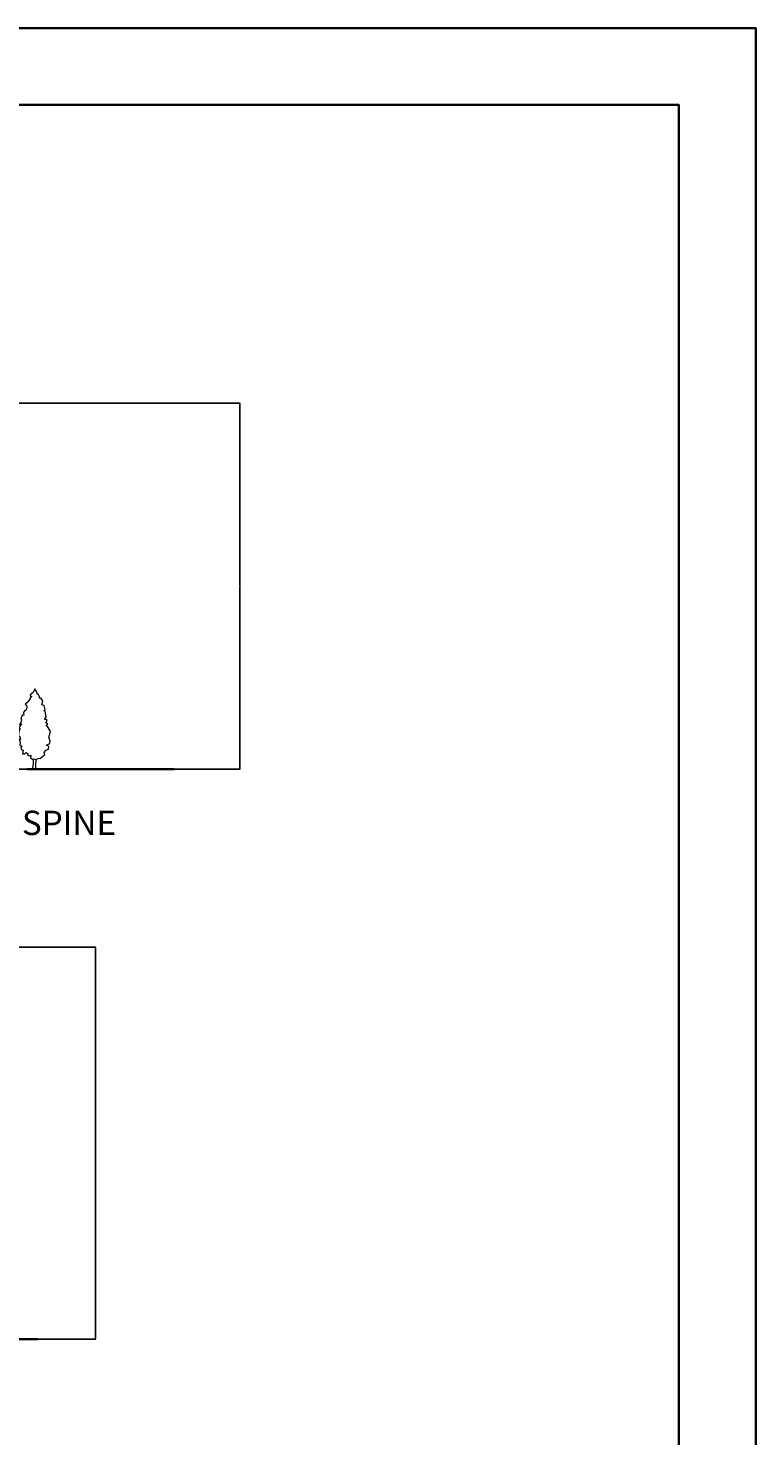
# Model space of a CAD drawing. Units: inches. Extents: x -934 to 898, y -1502 to 444.
# Tile 10 of 10: x 286 to 898, y -739 to 444. Entities that reach past the tile are written whole.
import ezdxf

# ---------------------------------------------------------------- set-up
doc = ezdxf.new("R2010")
doc.units = ezdxf.units.IN
doc.header["$MEASUREMENT"] = 0
for name, color, linetype, lineweight in [('A-ANNO-DIMS', 2, 'Continuous', 18), ('A-ANNO-TITL', 7, 'Continuous', 30), ('A-ANNO-TTLB', 7, 'Continuous', 35), ('L-GRND', 7, 'Continuous', 35), ('L-PLNT-TREE', 3, 'Continuous', 13)]:
    doc.layers.add(name, color=color, linetype=linetype, lineweight=lineweight)
doc.styles.get("Standard").update_dxf_attribs({"font": 'arial.ttf'})
doc.dimstyles.get("Standard").update_dxf_attribs({"dimtxt": 0.18, "dimasz": 0.18, "dimexe": 0.18, "dimexo": 0.0625, "dimgap": 0.09, "dimtad": 0, "dimtih": 1, "dimtoh": 1, "dimdec": 4, "dimzin": 0, "dimdsep": 46, "dimtxsty": 'Standard', "dimcen": 0.09, "dimadec": 0, "dimazin": 0, "dimtfac": 1, "dimtdec": 4, "dimtofl": 0, "dimtmove": 0, "dimatfit": 3, "dimfxl": 1, "dimtolj": 1, "dimtzin": 0, "dimarcsym": 0})

# ---------------------------------------------------------------- blocks, each defined once
blk = doc.blocks.new('*U5')
blk.add_lwpolyline([(-2.754, 191.699), (-6.78, 182.851), (-13.682, 176.953), (-11.956, 173.266), (-9.656, 172.529), (-14.257, 170.317), (-13.682, 167.368), (-21.733, 157.783), (-25.184, 154.834), (-21.158, 150.41), (-21.733, 147.461), (-22.884, 140.825), (-26.334, 140.087), (-29.21, 134.926), (-28.635, 129.028), (-32.661, 128.291), (-36.111, 120.18), (-34.386, 118.706), (-35.536, 111.333), (-38.987, 106.171), (-34.386, 107.646), (-40.712, 98.798), (-37.261, 95.849), (-40.712, 90.688), (-41.287, 80.366), (-38.412, 78.154), (-36.686, 70.781), (-39.562, 71.518), (-37.261, 64.145), (-38.412, 57.509), (-36.111, 58.247), (-33.236, 52.348), (-35.536, 53.086), (-34.961, 46.45), (-30.36, 44.975), (-31.51, 36.128), (-26.334, 36.865), (-23.459, 39.814), (-18.283, 36.128), (-20.008, 33.178), (-14.832, 31.704), (-11.956, 33.178), (-12.531, 27.28), (-6.205, 22.856), (-3.905, 24.331), (0.121, 22.856), (8.173, 26.543), (11.624, 25.068), (12.199, 27.28), (21.4, 34.653), (19.675, 39.077), (23.701, 44.975), (30.027, 47.924), (30.602, 53.823), (25.426, 56.772), (32.903, 61.196), (34.053, 67.094), (30.602, 75.205), (34.628, 89.951), (26.576, 103.222), (23.701, 103.222), (28.302, 107.646), (23.701, 110.595), (26.576, 115.756), (25.426, 117.968), (20.825, 118.706), (24.276, 124.604), (22.551, 137.876), (19.1, 139.35), (22.551, 140.825), (19.675, 151.884), (14.499, 153.359), (16.224, 162.207), (12.199, 170.317), (10.473, 167.368), (5.872, 179.165), (4.147, 177.69), (0.696, 187.275), (-0.454, 185.8)], close=True)
for points in [[(-6.813, 23.669), (-6.813, 11.669), (-8.627, 0)], [(0.387, 23.669), (-0.576, 13.271), (-0.576, 3.686), (0, 0)]]:
    blk.add_lwpolyline(points)
blk = doc.blocks.new('*D80')
at = {"layer": 'A-ANNO-DIMS', "color": 0, "lineweight": -2, "transparency": 16777216}
for p, q in [((261.6, 129.1), (464.3, 129.1)), ((464.1, 128.9), (464.1, -24.6)), ((464.1, -178.5), (464.1, -25)), ((239.7, -178.7), (464.3, -178.7))]:
    blk.add_line(p, q, dxfattribs=at)
at = {"layer": 'A-ANNO-DIMS', "color": 0, "transparency": 16777216}
for points in [[(464.1, 128.9), (464.2, 128.9), (464.1, 129.1)], [(464.1, -178.5), (464.2, -178.5), (464.1, -178.7)]]:
    blk.add_solid(points, dxfattribs=at)
at = {"layer": 'Defpoints', "color": 0, "transparency": 16777216}
for p in [(261.6, 129.1), (464.1, 129.1), (239.6, -178.7)]:
    blk.add_point(p, dxfattribs=at)
at = {"layer": 'A-ANNO-DIMS', "color": 0, "transparency": 16777216, "insert": (464.1, -24.8), "char_height": 0.18, "attachment_point": 5}
blk.add_mtext('\\A1;307.8', dxfattribs=at)
blk = doc.blocks.new('*D98')
at = {"layer": 'A-ANNO-DIMS', "color": 0, "lineweight": -2, "transparency": 16777216}
for p, q in [((176.3, -328.5), (343, -328.5)), ((342.8, -328.7), (342.8, -493.1)), ((342.8, -657.8), (342.8, -493.4)), ((190.1, -658), (343, -658))]:
    blk.add_line(p, q, dxfattribs=at)
at = {"layer": 'A-ANNO-DIMS', "color": 0, "transparency": 16777216}
for points in [[(342.8, -328.7), (342.9, -328.7), (342.8, -328.5)], [(342.8, -657.8), (342.9, -657.8), (342.8, -658)]]:
    blk.add_solid(points, dxfattribs=at)
at = {"layer": 'Defpoints', "color": 0, "transparency": 16777216}
for p in [(176.3, -328.5), (342.8, -328.5), (190, -658)]:
    blk.add_point(p, dxfattribs=at)
at = {"layer": 'A-ANNO-DIMS', "color": 0, "transparency": 16777216, "insert": (342.8, -493.3), "char_height": 0.18, "attachment_point": 5}
blk.add_mtext('\\A1;329.5', dxfattribs=at)

msp = doc.modelspace()

# ---------------------------------------------------------------- linework, layer by layer
at = {"layer": 'A-ANNO-TTLB'}
for points in [[(-933.5092, 444.4646), (897.7239, 444.4646), (897.7239, -1501.5858), (-933.5092, -1501.5858)], [(-892.081, 380.0228), (832.9871, 380.0228), (832.9871, -1448.0237), (-892.081, -1448.0237)]]:
    msp.add_lwpolyline(points, close=True, dxfattribs=at)
at = {"layer": 'L-GRND'}
for p, q in [((284.8904, -178.6804), (408.8772, -178.6804)), ((190.0344, -658.003), (294.2707, -658.003))]:
    msp.add_line(p, q, dxfattribs=at)

# ---------------------------------------------------------------- block references
at = {"layer": 'L-PLNT-TREE', "xscale": 0.3528399638811642, "yscale": 0.3528399638811642, "zscale": 0.3528399638811642}
msp.add_blockref('*U5', (292.566, -178.7166), dxfattribs=at)

# ---------------------------------------------------------------- texts
at = {"layer": 'A-ANNO-TITL'}
msp.add_text('LINEAR   CAMPUS   AXIS ELEVATION   RESEARCH   AND   INNOVATION   SPINE ', height=20.457511, dxfattribs=at).set_placement((-613.4854, -234.1138))

# ---------------------------------------------------------------- dimensions: what is measured, and where the dimension line sits
at = {"layer": 'A-ANNO-DIMS'}
for base, p1, p2, picture, middle in [((464.1272, 129.1024), (239.6401, -178.6804), (261.5611, 129.1024), '*D80', (464.1272, -24.789)), ((342.8207, -328.5269), (190.0344, -658.003), (176.286, -328.5269), '*D98', (342.8207, -493.265))]:
    dim = msp.add_linear_dim(base=base, p1=p1, p2=p2, angle=90, dimstyle='Standard', override={"dimdec": 1, "dimlfac": 1, "dimrnd": 0, "dimzin": 0, "dimdsep": 46, "dimlunit": 2}, dxfattribs=at)
    dim.commit()
    dim.dimension.update_dxf_attribs({"geometry": picture, "text_midpoint": middle})

doc.saveas('drawing.dxf')
